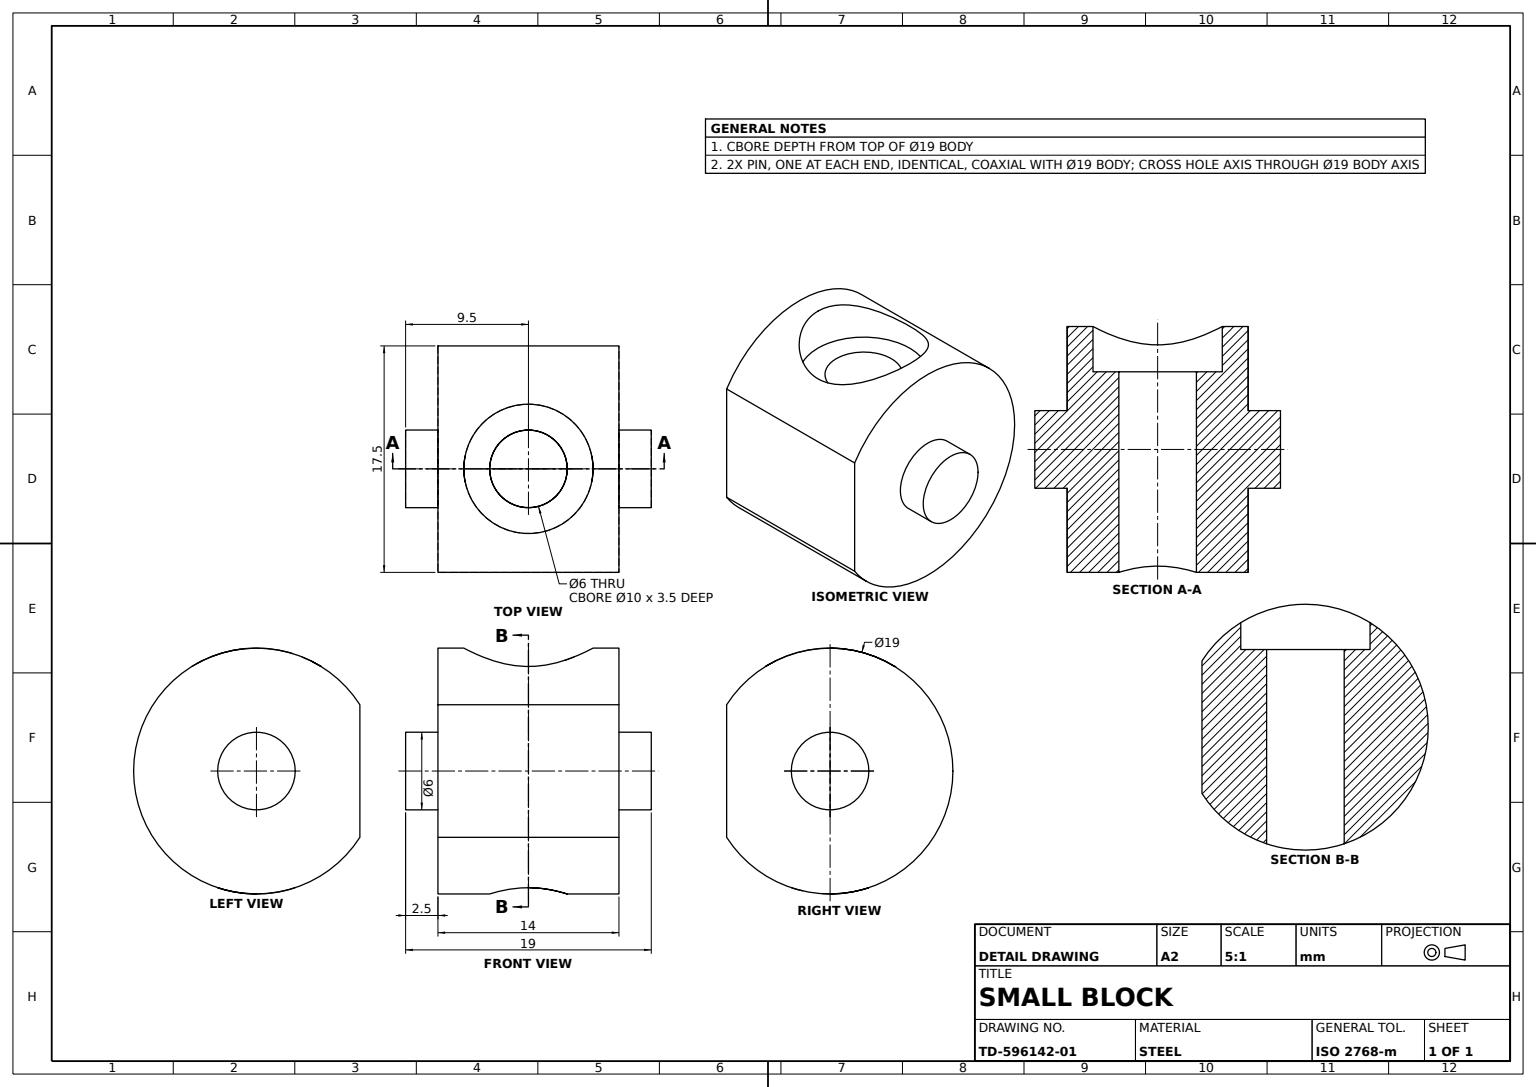
SolidWorks part; units mm, degrees
material "Plain Carbon Steel"
ref_plane "Front Plane" through (0, 0, 0) normal (0, 0, 1) x (1, 0, 0)
ref_plane "Top Plane" through (0, 0, 0) normal (0, 1, 0) x (1, 0, 0)
ref_plane "Right Plane" through (0, 0, 0) normal (1, 0, 0) x (0, 0, -1)
sketch "Body Profile Ø19 D-Flat" plane through (0, 0, 0) normal (0, 0, 1) x (1, 0, 0)
  line L0 (8, 5.1235) -> (8, -5.1235)
  arc A0 (8, 5.1235) -> (8, -5.1235) centre (0, 0) ccw
  dimension "D1" = 19
  dimension "D2" = 10.247
extrude "Bushing Body" add sketch "Body Profile Ø19 D-Flat" along normal blind 14
sketch "Front Pivot Pin Profile Ø6" plane through (0, 0, 14) normal (0, 0, 1) x (1, 0, 0)
  circle A0 centre (0, 0) radius 3
  dimension "D1" = 6
extrude "Front Pivot Pin Ø6" add sketch "Front Pivot Pin Profile Ø6" along normal blind 2.5
sketch "Rear Pivot Pin Profile Ø6" plane through (0, 0, 0) normal (0, 0, -1) x (-1, 0, 0)
  circle A0 centre (0, 0) radius 3
  dimension "D1" = 6
extrude "Rear Pivot Pin Ø6" add sketch "Rear Pivot Pin Profile Ø6" along normal blind 2.5
ref_plane "Plane1" through (0, 10, 0) normal (0, 1, 0) x (1, 0, 0)
sketch "Cross Counterbore Profile" plane through (0, 10, 0) normal (0, 1, 0) x (1, 0, 0)
  line L0 (8, -14) -> (8, 0) construction
  line L1 (3, 2.5) -> (-3, 2.5) construction
  circle A0 centre (0, -7) radius 5
  dimension "D1" = 10
  dimension "D2" = 8
  dimension "D3" = 9.5
extrude "Cross Counterbore" cut sketch "Cross Counterbore Profile" against normal blind 4
sketch "Cross Hole Profile Ø6" plane through (0, 6, 0) normal (0, 1, 0) x (1, 0, 0)
  circle A0 centre (0, -7) radius 3
  dimension "D1" = 6
extrude "Cross Hole Ø6" cut sketch "Cross Hole Profile Ø6" against normal blind 16
